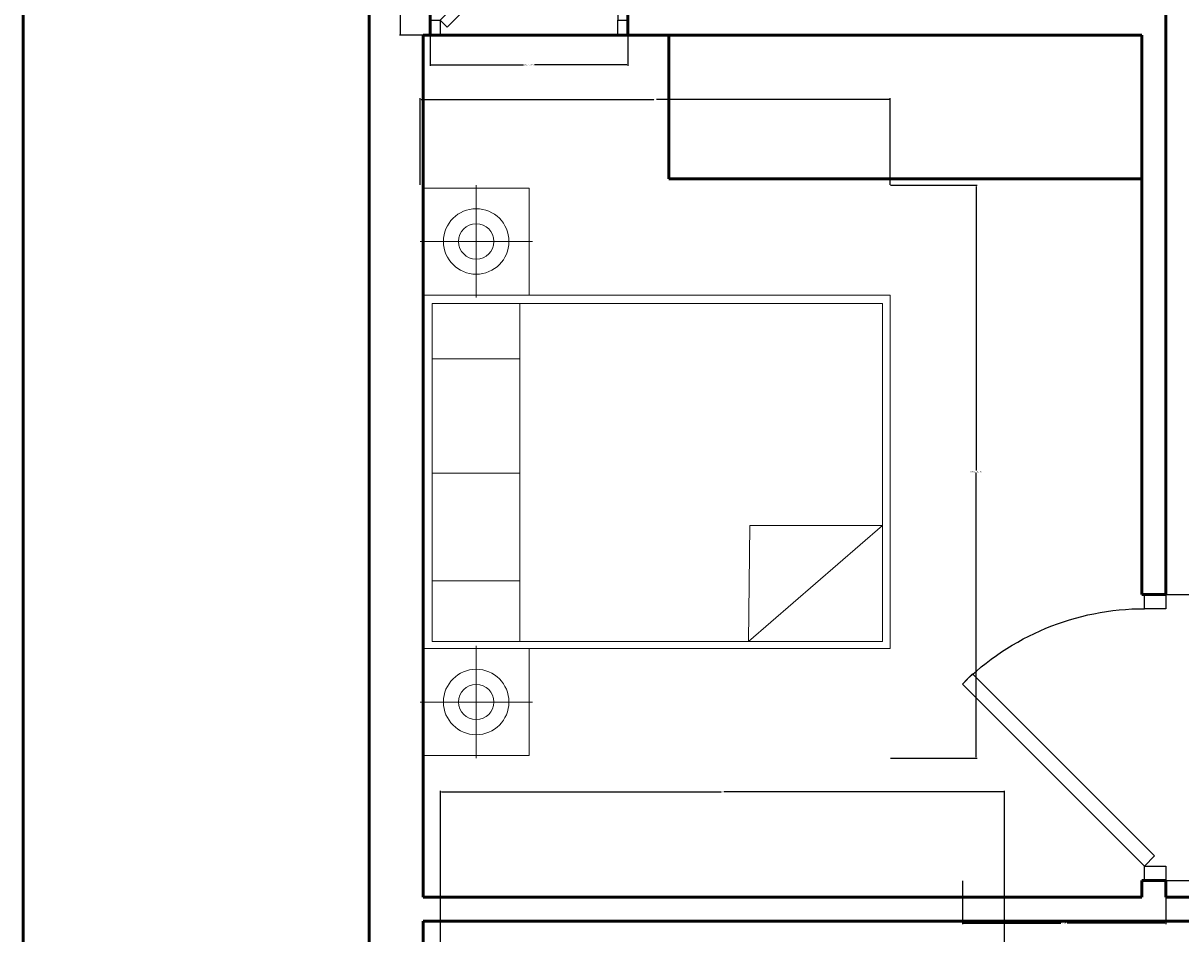
# Model space of a CAD drawing. Units: inches. Extents: x 64 to 1167, y 117 to 939.
# Tile 3 of 56: x 64 to 258, y 431 to 583. Entities that reach past the tile are written whole.
import ezdxf

# ---------------------------------------------------------------- set-up
doc = ezdxf.new("R2010")
doc.units = ezdxf.units.IN
doc.header["$MEASUREMENT"] = 0
for name, color, linetype, lineweight in [('A-ANNO-DIMS', 2, 'Continuous', 18), ('A-ANNO-TTLB', 7, 'Continuous', 50), ('A-DOOR', 4, 'Continuous', 25), ('A-FURN', 8, 'Continuous', 18), ('A-WALL', 7, 'Continuous', 50)]:
    doc.layers.add(name, color=color, linetype=linetype, lineweight=lineweight)
doc.styles.get("Standard").update_dxf_attribs({"font": 'arial.ttf'})
doc.dimstyles.get("Standard").update_dxf_attribs({"dimtxt": 0.18, "dimasz": 0.18, "dimexe": 0.18, "dimexo": 0.0625, "dimgap": 0.09, "dimtad": 0, "dimtih": 1, "dimtoh": 1, "dimdec": 4, "dimzin": 0, "dimdsep": 46, "dimtxsty": 'Standard', "dimcen": 0.09, "dimadec": 0, "dimazin": 0, "dimtfac": 1, "dimtdec": 4, "dimtofl": 0, "dimtmove": 0, "dimatfit": 3, "dimfxl": 1, "dimtolj": 1, "dimtzin": 0, "dimarcsym": 0})

# ---------------------------------------------------------------- blocks, each defined once
blk = doc.blocks.new('A$C68901CC0')
for p, q in [((10.95, 26.62), (12.35, 28.01)), ((12.35, 28.01), (37.4, 2.95)), ((36.01, 1.56), (10.95, 26.62)), ((0, 2.95), (0, 0)), ((1.97, 2.95), (0, 2.95)), ((1.97, 0), (1.97, 2.95)), ((37.4, 2.95), (36.01, 1.56)), ((37.4, 2.95), (37.4, 0)), ((39.37, 2.95), (37.4, 2.95)), ((39.37, 0), (39.37, 2.95)), ((0, 0), (1.97, 0)), ((37.4, 0), (39.37, 0))]:
    blk.add_line(p, q)
blk.add_arc((37.4, 2.95), 35.43, 135, 180)
blk = doc.blocks.new('A$C214F6537')
for p, q in [((0.0183, 0.07795, -0.00664), (0.00043, 0.07795, -0.00664)), ((0.00043, 0.07795, -0.00664), (0.00043, 0.06024, -0.00664)), ((0.00043, 0.07795, -0.00664), (0.09523, 0.07795, -0.00664)), ((0.00043, 0.06024, -0.00664), (0.00043, 0.07795, -0.00664)), ((0.00937, 0.06911, -0.01727), (0.00937, 0.07848, -0.01727)), ((0.0183, 0, -0.00664), (0.0183, 0.07795, -0.00664)), ((0.0183, 0.07795, -0.00664), (0.07735, 0.07795, -0.00664)), ((0.0183, 0.06024, -0.00664), (0.0183, 0.07795, -0.00664)), ((0.07735, 0.07795, -0.00664), (0.07735, 0, -0.00664)), ((0.09523, 0.07795, -0.00664), (0.07735, 0.07795, -0.00664)), ((0.07735, 0.07795, -0.00664), (0.07735, 0.06024, -0.00664)), ((0.0863, 0.06911, -0.01727), (0.0863, 0.07848, -0.01727)), ((0.09523, 0.06024, -0.00664), (0.09523, 0.07795, -0.00664)), ((0.09523, 0.07795, -0.00664), (0.09523, 0.06024, -0.00664)), ((0.01949, 0.07644, -0.00664), (0.07594, 0.07644, -0.00664)), ((0.01949, 0.06182, -0.00664), (0.01949, 0.07644, -0.00664)), ((0.02963, 0.07644, -0.00664), (0.02963, 0.06182, -0.00664)), ((0.04759, 0.07644, -0.00664), (0.04759, 0.06182, -0.00664)), ((0.0667, 0.07644, -0.00664), (0.0667, 0.06182, -0.00664)), ((0.07594, 0.07644, -0.00664), (0.07594, 0.06182, -0.00664)), ((0.00937, 0.06911, -0.01727), (0, 0.06911, -0.01727)), ((0.00937, 0.06911, -0.01727), (0.00937, 0.05973, -0.01727)), ((0.00937, 0.06911, -0.01727), (0.01875, 0.06911, -0.01727)), ((0.0863, 0.06911, -0.01727), (0.07693, 0.06911, -0.01727)), ((0.0863, 0.06911, -0.01727), (0.09568, 0.06911, -0.01727)), ((0.0863, 0.06911, -0.01727), (0.0863, 0.05973, -0.01727)), ((0.00043, 0.06024, -0.00664), (0.0183, 0.06024, -0.00664)), ((0.0183, 0.06024, -0.00664), (0.00043, 0.06024, -0.00664)), ((0.0183, 0, -0.00664), (0.0183, 0.06024, -0.00664)), ((0.01949, 0.00127, -0.00664), (0.01949, 0.06182, -0.00664)), ((0.07594, 0.06182, -0.00664), (0.01949, 0.06182, -0.00664)), ((0.07594, 0.06182, -0.00664), (0.07594, 0.00127, -0.00664)), ((0.07735, 0.06024, -0.00664), (0.09523, 0.06024, -0.00664)), ((0.09523, 0.06024, -0.00664), (0.07735, 0.06024, -0.00664)), ((0.07735, 0.06024, -0.00664), (0.07735, 0, -0.00664)), ((0.01949, 0.02364, -0.00664), (0.03887, 0.00127, -0.00664)), ((0.03887, 0.02341, -0.00664), (0.01949, 0.02364, -0.00664)), ((0.03887, 0.00127, -0.00664), (0.03887, 0.02341, -0.00664)), ((0.07735, 0, -0.00664), (0.0183, 0, -0.00664)), ((0.07735, 0, -0.00664), (0.0183, 0, -0.00664)), ((0.07594, 0.00127, -0.00664), (0.01949, 0.00127, -0.00664))]:
    blk.add_line(p, q)
for centre, radius in [((0.00937, 0.06911, -0.01727), 0.00547), ((0.0863, 0.06911, -0.01727), 0.00547), ((0.00937, 0.06911, -0.01727), 0.00295), ((0.0863, 0.06911, -0.01727), 0.00295)]:
    blk.add_circle(centre, radius)
blk = doc.blocks.new('*D58')
at = {"layer": 'A-ANNO-DIMS', "color": 0, "lineweight": -2, "transparency": 16777216}
for p, q in [((255.17, 487.78), (262.45, 487.78)), ((262.27, 487.6), (262.27, 464.08)), ((262.27, 440.19), (262.27, 463.71)), ((255.17, 440.01), (262.45, 440.01))]:
    blk.add_line(p, q, dxfattribs=at)
for points in [[(262.24, 487.6), (262.3, 487.6), (262.27, 487.78)], [(262.24, 440.19), (262.3, 440.19), (262.27, 440.01)]]:
    blk.add_solid(points, dxfattribs=at)
at = {"layer": 'Defpoints', "color": 0, "lineweight": -2, "transparency": 16777216}
for p in [(255.11, 487.78), (255.11, 440.01), (262.27, 440.01)]:
    blk.add_point(p, dxfattribs=at)
at = {"layer": 'A-ANNO-DIMS', "color": 0, "transparency": 16777216, "insert": (262.27, 463.9), "char_height": 0.18, "attachment_point": 5}
blk.add_mtext('\\A1;DOOR 48 TYP.', dxfattribs=at)
blk = doc.blocks.new('*D59')
at = {"layer": 'A-ANNO-DIMS', "color": 0, "lineweight": -2, "transparency": 16777216}
for p, q in [((221.13, 439.95), (221.13, 432.67)), ((255.11, 439.95), (255.11, 432.67)), ((221.31, 432.85), (237.59, 432.85)), ((254.93, 432.85), (238.64, 432.85))]:
    blk.add_line(p, q, dxfattribs=at)
for points in [[(221.31, 432.88), (221.31, 432.82), (221.13, 432.85)], [(254.93, 432.88), (254.93, 432.82), (255.11, 432.85)]]:
    blk.add_solid(points, dxfattribs=at)
at = {"layer": 'Defpoints', "color": 0, "lineweight": -2, "transparency": 16777216}
for p in [(221.13, 440.01), (255.11, 440.01), (221.13, 432.85)]:
    blk.add_point(p, dxfattribs=at)
at = {"layer": 'A-ANNO-DIMS', "color": 0, "transparency": 16777216, "insert": (238.12, 432.85), "char_height": 0.18, "attachment_point": 5}
blk.add_mtext('\\A1;34 TYP.', dxfattribs=at)
blk = doc.blocks.new('*D60')
at = {"layer": 'A-ANNO-DIMS', "color": 0, "lineweight": -2, "transparency": 16777216}
for p, q in [((132.28, 581.14), (132.28, 576.07)), ((165.28, 581.14), (165.28, 576.07)), ((132.46, 576.25), (147.84, 576.25)), ((165.1, 576.25), (149.71, 576.25))]:
    blk.add_line(p, q, dxfattribs=at)
for points in [[(132.46, 576.28), (132.46, 576.22), (132.28, 576.25)], [(165.1, 576.28), (165.1, 576.22), (165.28, 576.25)]]:
    blk.add_solid(points, dxfattribs=at)
at = {"layer": 'Defpoints', "color": 0, "lineweight": -2, "transparency": 16777216}
for p in [(132.28, 581.2), (165.28, 581.2), (132.28, 576.25)]:
    blk.add_point(p, dxfattribs=at)
at = {"layer": 'A-ANNO-DIMS', "color": 0, "transparency": 16777216, "insert": (148.78, 576.25), "char_height": 0.18, "attachment_point": 5}
blk.add_mtext('\\A1;DOOR 33 TYP.', dxfattribs=at)
blk = doc.blocks.new('*D61')
at = {"layer": 'A-ANNO-DIMS', "color": 0, "lineweight": -2, "transparency": 16777216}
for p, q in [((132.21, 604.68), (127.15, 604.68)), ((127.33, 604.5), (127.33, 593.12)), ((127.33, 581.38), (127.33, 592.76)), ((132.21, 581.2), (127.15, 581.2))]:
    blk.add_line(p, q, dxfattribs=at)
for points in [[(127.3, 604.5), (127.36, 604.5), (127.33, 604.68)], [(127.3, 581.38), (127.36, 581.38), (127.33, 581.2)]]:
    blk.add_solid(points, dxfattribs=at)
at = {"layer": 'Defpoints', "color": 0, "lineweight": -2, "transparency": 16777216}
for p in [(127.33, 604.68), (132.28, 604.68), (132.28, 581.2)]:
    blk.add_point(p, dxfattribs=at)
at = {"layer": 'A-ANNO-DIMS', "color": 0, "transparency": 16777216, "insert": (127.33, 592.94), "char_height": 0.18, "attachment_point": 5}
blk.add_mtext('\\A1;23 TYP.', dxfattribs=at)
blk = doc.blocks.new('*D80')
at = {"layer": 'A-ANNO-DIMS', "color": 0, "lineweight": -2, "transparency": 16777216}
for p, q in [((209.12, 556.11), (223.59, 556.11)), ((223.41, 555.93), (223.41, 508.45)), ((223.41, 460.61), (223.41, 508.09)), ((209.12, 460.43), (223.59, 460.43))]:
    blk.add_line(p, q, dxfattribs=at)
for points in [[(223.38, 555.93), (223.44, 555.93), (223.41, 556.11)], [(223.38, 460.61), (223.44, 460.61), (223.41, 460.43)]]:
    blk.add_solid(points, dxfattribs=at)
at = {"layer": 'Defpoints', "color": 0, "lineweight": -2, "transparency": 16777216}
for p in [(209.06, 556.11), (223.41, 556.11), (209.06, 460.43)]:
    blk.add_point(p, dxfattribs=at)
at = {"layer": 'A-ANNO-DIMS', "color": 0, "transparency": 16777216, "insert": (223.41, 508.27), "char_height": 0.18, "attachment_point": 5}
blk.add_mtext('\\A1;DOUBLE BED 96', dxfattribs=at)
blk = doc.blocks.new('*D81')
at = {"layer": 'A-ANNO-DIMS', "color": 0, "lineweight": -2, "transparency": 16777216}
for p, q in [((130.58, 556.17), (130.58, 570.64)), ((130.76, 570.46), (169.6, 570.46)), ((208.88, 570.46), (170.04, 570.46)), ((209.06, 556.17), (209.06, 570.64))]:
    blk.add_line(p, q, dxfattribs=at)
for points in [[(130.76, 570.49), (130.76, 570.43), (130.58, 570.46)], [(208.88, 570.49), (208.88, 570.43), (209.06, 570.46)]]:
    blk.add_solid(points, dxfattribs=at)
at = {"layer": 'Defpoints', "color": 0, "lineweight": -2, "transparency": 16777216}
for p in [(130.58, 570.46), (130.58, 556.11), (209.06, 556.11)]:
    blk.add_point(p, dxfattribs=at)
at = {"layer": 'A-ANNO-DIMS', "color": 0, "transparency": 16777216, "insert": (169.82, 570.46), "char_height": 0.18, "attachment_point": 5}
blk.add_mtext('\\A1;78', dxfattribs=at)
blk = doc.blocks.new('*D83')
at = {"layer": 'A-ANNO-DIMS', "color": 0, "lineweight": -2, "transparency": 16777216}
for p, q in [((133.97, 429.63), (133.97, 454.99)), ((134.15, 454.81), (180.86, 454.81)), ((228.01, 454.81), (181.3, 454.81)), ((228.19, 429.63), (228.19, 454.99))]:
    blk.add_line(p, q, dxfattribs=at)
for points in [[(134.15, 454.84), (134.15, 454.78), (133.97, 454.81)], [(228.01, 454.84), (228.01, 454.78), (228.19, 454.81)]]:
    blk.add_solid(points, dxfattribs=at)
at = {"layer": 'Defpoints', "color": 0, "lineweight": -2, "transparency": 16777216}
for p in [(133.97, 454.81), (133.97, 429.56), (228.19, 429.56)]:
    blk.add_point(p, dxfattribs=at)
at = {"layer": 'A-ANNO-DIMS', "color": 0, "transparency": 16777216, "insert": (181.08, 454.81), "char_height": 0.18, "attachment_point": 5}
blk.add_mtext('\\A1;94', dxfattribs=at)

msp = doc.modelspace()

# ---------------------------------------------------------------- linework, layer by layer
at = {"layer": 'A-ANNO-TTLB'}
msp.add_lwpolyline([(64.31, 939.22), (512.77, 939.22), (512.77, 116.55), (64.31, 116.55)], close=True, dxfattribs=at)
at = {"layer": 'A-WALL'}
for p, q in [((122.11, 863.2), (122.11, 155.2)), ((132.28, 585.2), (132.28, 581.2)), ((165.28, 585.2), (165.28, 581.2)), ((255.11, 585.2), (255.11, 487.78)), ((131.11, 581.2), (131.11, 437.2)), ((251.11, 581.2), (131.11, 581.2)), ((172.14, 581.2), (172.14, 557.2)), ((251.11, 581.2), (251.11, 487.78)), ((251.11, 557.2), (172.14, 557.2)), ((251.11, 487.78), (255.11, 487.78)), ((251.11, 440.01), (255.11, 440.01)), ((251.11, 440.01), (251.11, 437.2)), ((255.11, 440.01), (255.11, 437.2)), ((251.11, 437.2), (131.11, 437.2)), ((279.11, 437.2), (255.11, 437.2)), ((131.11, 433.2), (131.11, 241.2)), ((279.11, 433.2), (131.11, 433.2))]:
    msp.add_line(p, q, dxfattribs=at)

# ---------------------------------------------------------------- block references
at = {"layer": 'A-DOOR', "xscale": -0.8381879042225197, "yscale": 0.8381879042225197, "zscale": 0.8381879042225197}
msp.add_blockref('A$C68901CC0', (165.28, 581.2), dxfattribs=at)
at = {"layer": 'A-DOOR', "xscale": -1.213305874571074, "yscale": 1.213305874571074, "zscale": 1.213305874571074, "rotation": 90}
msp.add_blockref('A$C68901CC0', (255.11, 487.78), dxfattribs=at)
at = {"layer": 'A-FURN', "xscale": 1000, "yscale": 1000, "zscale": 1000, "rotation": 90}
msp.add_blockref('A$C214F6537', (209.06, 460.43, 6.64), dxfattribs=at)

# ---------------------------------------------------------------- dimensions: what is measured, and where the dimension line sits
at = {"layer": 'A-ANNO-DIMS'}
for base, p1, p2, angle, text, picture, middle in [((127.33, 604.68), (132.28, 581.2), (132.28, 604.68), 90, '<> TYP.', '*D61', (127.33, 592.94)), ((132.28, 576.25), (165.28, 581.2), (132.28, 581.2), 180, 'DOOR <> TYP.', '*D60', (148.78, 576.25)), ((223.41, 556.11), (209.06, 460.43), (209.06, 556.11), 90, 'DOUBLE BED <>', '*D80', (223.41, 508.27)), ((262.27, 440.01), (255.11, 487.78), (255.11, 440.01), 270, 'DOOR <> TYP.', '*D58', (262.27, 463.9)), ((221.13, 432.85), (255.11, 440.01), (221.13, 440.01), 180, '<> TYP.', '*D59', (238.12, 432.85))]:
    dim = msp.add_linear_dim(base=base, p1=p1, p2=p2, angle=angle, text=text, dimstyle='Standard', override={"dimdec": 0, "dimlfac": 1, "dimrnd": 0, "dimzin": 0, "dimdsep": 46, "dimlunit": 2}, dxfattribs=at)
    dim.commit()
    dim.dimension.update_dxf_attribs({"geometry": picture, "text_midpoint": middle})
for base, p1, p2, picture, middle in [((130.58, 570.46), (209.06, 556.11), (130.58, 556.11), '*D81', (169.82, 570.46)), ((133.97, 454.81), (228.19, 429.56), (133.97, 429.56), '*D83', (181.08, 454.81))]:
    dim = msp.add_linear_dim(base=base, p1=p1, p2=p2, angle=180, dimstyle='Standard', override={"dimdec": 0, "dimlfac": 1, "dimrnd": 0, "dimzin": 0, "dimdsep": 46, "dimlunit": 2}, dxfattribs=at)
    dim.commit()
    dim.dimension.update_dxf_attribs({"geometry": picture, "text_midpoint": middle})

doc.saveas('drawing.dxf')
